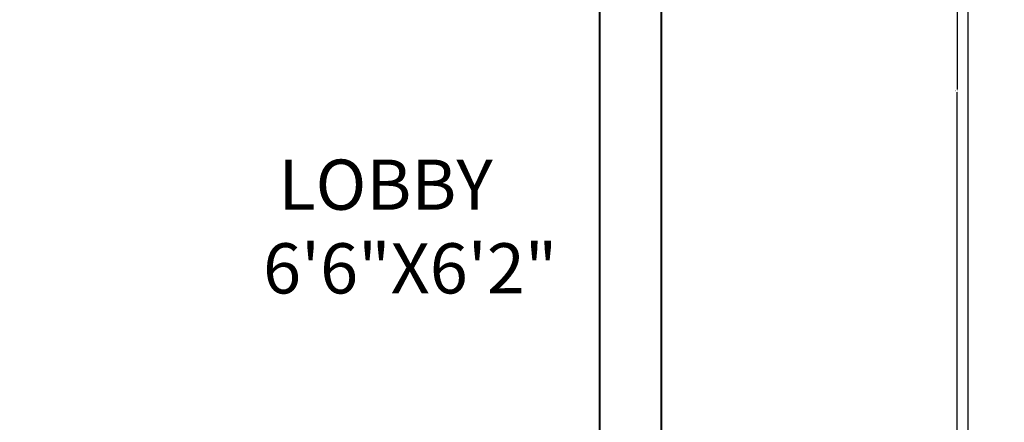
# Model space of a CAD drawing. Units: inches. Extents: x 182 to 1022, y -617 to 111.
# Tile 27 of 33: x 879 to 1022, y -395 to -337. Entities that reach past the tile are written whole.
import ezdxf

# ---------------------------------------------------------------- set-up
doc = ezdxf.new("R2010")
doc.units = ezdxf.units.IN
doc.header["$MEASUREMENT"] = 0
for name, color, linetype, lineweight in [('A-ANNO-DIMS', 2, 'Continuous', 18), ('A-AREA-IDEN', 8, 'Continuous', 18), ('wall', 1, 'Continuous', 40)]:
    doc.layers.add(name, color=color, linetype=linetype, lineweight=lineweight)
doc.styles.get("Standard").update_dxf_attribs({"font": 'arial.ttf'})
doc.dimstyles.get("Standard").update_dxf_attribs({"dimtxt": 0.18, "dimasz": 0.18, "dimexe": 0.18, "dimexo": 0.0625, "dimgap": 0.09, "dimtad": 0, "dimtih": 1, "dimtoh": 1, "dimdec": 1, "dimzin": 0, "dimdsep": 46, "dimlunit": 4, "dimtxsty": 'Standard', "dimcen": 0.09, "dimadec": 0, "dimazin": 0, "dimtfac": 1, "dimtdec": 1, "dimtofl": 0, "dimtmove": 0, "dimatfit": 3, "dimfxl": 1, "dimtolj": 1, "dimtzin": 0, "dimarcsym": 0})

# ---------------------------------------------------------------- blocks, each defined once
blk = doc.blocks.new('_ArchTick')
at = {"color": 0, "linetype": 'ByBlock', "const_width": 0.15}
blk.add_lwpolyline([(-0.5, -0.5), (0.5, 0.5)], dxfattribs=at)
blk = doc.blocks.new('*D8')
at = {"layer": 'A-ANNO-DIMS', "color": 0, "lineweight": -2, "transparency": 16777216}
for p, q in [((1016.69, -0.37), (1016.69, -260.42)), ((1016.69, -540.37), (1016.69, -280.32))]:
    blk.add_line(p, q, dxfattribs=at)
at = {"layer": 'Defpoints', "color": 0, "transparency": 16777216}
for p in [(972.3, -0.37), (972.3, -540.37), (1016.69, -540.37)]:
    blk.add_point(p, dxfattribs=at)
at = {"layer": 'A-ANNO-DIMS', "color": 0, "lineweight": -2, "transparency": 16777216, "xscale": 8, "yscale": 8, "zscale": 8}
for p, rotation in [((1016.69, -0.37), 90), ((1016.69, -540.37), 270)]:
    blk.add_blockref('_ArchTick', p, dxfattribs=dict(at, rotation=rotation))
at = {"layer": 'A-ANNO-DIMS', "color": 0, "transparency": 16777216, "insert": (1016.69, -270.37), "char_height": 8, "attachment_point": 5, "rotation": 90}
blk.add_mtext("\\A1;45'", dxfattribs=at)
blk = doc.blocks.new('*D39')
at = {"layer": 'A-ANNO-DIMS', "color": 0, "lineweight": -2, "transparency": 16777216}
for p, q in [((238.4, -288.54), (1015.28, -288.54)), ((1015.1, -288.72), (1015.1, -346.77)), ((1015.1, -405.19), (1015.1, -347.14)), ((238.43, -405.37), (1015.28, -405.37))]:
    blk.add_line(p, q, dxfattribs=at)
at = {"layer": 'A-ANNO-DIMS', "color": 0, "transparency": 16777216}
for points in [[(1015.07, -288.72), (1015.13, -288.72), (1015.1, -288.54)], [(1015.07, -405.19), (1015.13, -405.19), (1015.1, -405.37)]]:
    blk.add_solid(points, dxfattribs=at)
at = {"layer": 'Defpoints', "color": 0, "transparency": 16777216}
for p in [(238.34, -288.54), (1015.1, -288.54), (238.36, -405.37)]:
    blk.add_point(p, dxfattribs=at)
at = {"layer": 'A-ANNO-DIMS', "color": 0, "transparency": 16777216, "insert": (1015.1, -346.96), "char_height": 0.18, "attachment_point": 5}
blk.add_mtext('\\A1;9\'-9"', dxfattribs=at)

msp = doc.modelspace()

# ---------------------------------------------------------------- linework, layer by layer
at = {"layer": 'wall'}
for p, q in [((972.3, -540.37), (972.3, -0.37)), ((963.3, -322.87), (963.3, -531.37))]:
    msp.add_line(p, q, dxfattribs=at)

# ---------------------------------------------------------------- texts
at = {"layer": 'A-AREA-IDEN', "insert": (914.56, -356.9), "char_height": 7.2703, "attachment_point": 1}
msp.add_mtext_dynamic_manual_height_columns(' LOBBY      6\'6"X6\'2"', width=42.598, gutter_width=1.21, heights=[0], dxfattribs=at)

# ---------------------------------------------------------------- dimensions: what is measured, and where the dimension line sits
at = {"layer": 'A-ANNO-DIMS'}
for base, p1, p2, override, picture, middle in [((1016.69, -540.37), (972.3, -0.37), (972.3, -540.37), {"dimtxt": 8, "dimasz": 8, "dimgap": 3, "dimtih": 0, "dimblk1": 'ArchTick', "dimblk2": 'ArchTick', "dimsah": 1, "dimse1": 1, "dimse2": 1, "dimclrd": 0, "dimclre": 0, "dimclrt": 0}, '*D8', (1016.69, -270.37)), ((1015.1, -288.54), (238.36, -405.37), (238.34, -288.54), {"dimdec": 1, "dimlfac": 1, "dimrnd": 0, "dimzin": 1, "dimdsep": 46, "dimlunit": 4, "dimfrac": 2}, '*D39', (1015.1, -346.96))]:
    dim = msp.add_linear_dim(base=base, p1=p1, p2=p2, angle=90, dimstyle='Standard', override=override, dxfattribs=at)
    dim.commit()
    dim.dimension.update_dxf_attribs({"geometry": picture, "text_midpoint": middle})

doc.saveas('drawing.dxf')
